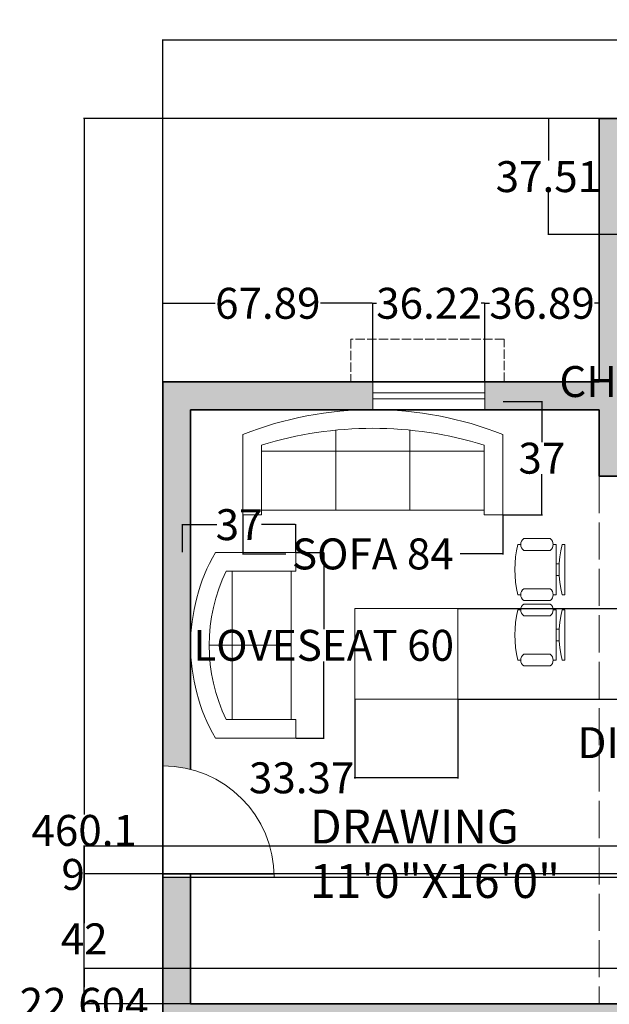
# Model space of a CAD drawing. Units: inches. Extents: x 143 to 746, y -392 to 145.
# Tile 2 of 6: x 143 to 334, y -173 to 145. Entities that reach past the tile are written whole.
import ezdxf

# ---------------------------------------------------------------- set-up
doc = ezdxf.new("R2010")
doc.units = ezdxf.units.IN
doc.header["$MEASUREMENT"] = 0
doc.linetypes.add('ACAD_ISO02W100', pattern=[15, 12, -3])
for name, color, linetype, lineweight in [('A-ANNO-DIMS', 2, 'Continuous', 18), ('A-AREA-IDEN', 7, 'Continuous', 20), ('A-DOOR', 3, 'Continuous', 18), ('A-FURN', 8, 'Continuous', 18), ('A-GLAZ', 4, 'Continuous', 18), ('A-GLAZ-OVHD', 4, 'ACAD_ISO02W100', 13), ('A-WALL', 7, 'Continuous', 35), ('A-WALL-OVHD', 7, 'ACAD_ISO02W100', 18)]:
    doc.layers.add(name, color=color, linetype=linetype, lineweight=lineweight)
doc.layers.add('A-WALL-PATT', color=252, linetype='Continuous', lineweight=13, true_color=0x939598)
doc.styles.get("Standard").update_dxf_attribs({"font": 'arial.ttf'})
doc.dimstyles.get("Standard").update_dxf_attribs({"dimtxt": 10, "dimasz": 0.18, "dimexe": 0.18, "dimexo": 0.0625, "dimgap": 0.09, "dimtad": 0, "dimtih": 1, "dimtoh": 1, "dimdec": 0, "dimzin": 0, "dimdsep": 46, "dimlunit": 3, "dimtxsty": 'Standard', "dimcen": 0.09, "dimadec": 0, "dimazin": 0, "dimtfac": 1, "dimtdec": 0, "dimtofl": 0, "dimtmove": 0, "dimatfit": 3, "dimfxl": 1, "dimtolj": 1, "dimtzin": 0, "dimarcsym": 0})

# ---------------------------------------------------------------- blocks, each defined once
blk = doc.blocks.new('Sofa - Roundback 7 ft.')
for p, q in [((-12.00002, -32.4421), (-12.00003, -6.5971)), ((11.99997, -32.4421), (11.99998, -6.5971)), ((-36.000027, -34), (-36.000027, -11.4696)), ((35.99998, -34), (35.99998, -11.4696)), ((-35.999844, -13.3819), (35.9998, -13.3819)), ((-36.000027, -32.4421), (35.99998, -32.4421))]:
    blk.add_line(p, q)
for points in [[(-36.000027, -34), (-42.000027, -34), (-42.000027, -8)], [(41.99998, -8), (41.99998, -34), (35.99998, -34)]]:
    blk.add_lwpolyline(points)
for centre, radius, start, end in [((0, -114.25), 114.25, 68.43141, 111.5686), ((-0.00001, -127.1968), 121.1968, 72.72033, 107.2797)]:
    blk.add_arc(centre, radius, start, end)
blk = doc.blocks.new('Sofa - Roundback Loveseat 5 ft.')
for p, q in [((0, -32.44198), (0, -5.99998)), ((-24, -33.99998), (-24, -11.46958)), ((24.00004, -33.99998), (24.00004, -11.46958)), ((-23.9998, -13.38178), (23.99986, -13.38178)), ((-24, -32.44198), (24.00004, -32.44198))]:
    blk.add_line(p, q)
for points in [[(-24, -33.99998), (-30, -33.99998), (-30, -7.99998)], [(30.00004, -7.99998), (30.00004, -33.99998), (24.00004, -33.99998)]]:
    blk.add_lwpolyline(points)
for centre, radius, start, end in [((0, -60.24998), 60.24998, 60.13715, 119.8628), ((0, -61.38438), 55.38444, 64.32083, 115.6792)]:
    blk.add_arc(centre, radius, start, end)
blk = doc.blocks.new('Chair - Desk')
for p, q in [((-8.5, 0), (-8.5, -1)), ((-8.5, 0), (8.5, 0)), ((8.5, 0), (8.5, -1)), ((-8.5, -3), (-8.5, -4)), ((-8.5, -3), (8.5, -3)), ((-2, -3), (-2, -1.9355)), ((2, -1.9576), (2, -3)), ((8.5, -3), (8.5, -4)), ((-10.5, -5), (-10.5, -14)), ((-6.5, -14), (-6.5, -5)), ((6.5, -5), (6.5, -14)), ((10.5, -14), (10.5, -5)), ((-8.5, -15), (-8.5, -16)), ((8.5, -15), (8.5, -16))]:
    blk.add_line(p, q)
for centre, radius, start, end in [((0, 34.625), 36.625, 256.5803, 283.4197), ((-8.5, -6.5), 2.5, 36.8699, 143.1301), ((8.5, -6.5), 2.5, 36.8699, 143.1301), ((-8.5, -12.5), 2.5, 216.8699, 323.1301), ((0, 19.625), 36.625, 256.5803, 283.4197), ((8.5, -12.5), 2.5, 216.8699, 323.1301)]:
    blk.add_arc(centre, radius, start, end)
blk = doc.blocks.new('DOOR-SINGLE-36IN')
for p, q in [((36, 36), (0, 36)), ((36, 35), (0, 35))]:
    blk.add_line(p, q)
blk.add_arc((36, 36), 36, 180, 270)
blk = doc.blocks.new('WINDOW-SHADE-49IN')
at = {"ltscale": 0.25}
for p, q in [((49.48, 13.79), (0, 13.79)), ((0, 13.79), (0, 0)), ((49.48, 0), (49.48, 13.79))]:
    blk.add_line(p, q, dxfattribs=at)
blk = doc.blocks.new('*D18')
at = {"layer": 'A-ANNO-DIMS', "color": 0, "lineweight": -2, "transparency": 16777216}
for p, q in [((426.49, 40.22), (410.54, 28.71)), ((428.36, 37.94), (426.53, 40.48)), ((412.12, 26.22), (410.29, 28.75)), ((410.25, 28.5), (410.07, 28.5)), ((410.4, 28.6), (410.25, 28.5))]:
    blk.add_line(p, q, dxfattribs=at)
at = {"layer": 'A-ANNO-DIMS', "color": 0, "transparency": 16777216}
for points in [[(426.47, 40.25), (426.51, 40.2), (426.64, 40.33)], [(410.53, 28.73), (410.56, 28.68), (410.4, 28.6)]]:
    blk.add_solid(points, dxfattribs=at)
at = {"layer": 'Defpoints', "color": 0, "transparency": 16777216}
for p in [(428.4, 37.89), (410.4, 28.6), (412.16, 26.17)]:
    blk.add_point(p, dxfattribs=at)
at = {"layer": 'A-ANNO-DIMS', "color": 0, "transparency": 16777216, "insert": (362.03, 28.5), "char_height": 10, "attachment_point": 5}
blk.add_mtext('\\A1;CHAIR 20 TYP.', dxfattribs=at)
blk = doc.blocks.new('*D28')
at = {"layer": 'A-ANNO-DIMS', "color": 0, "lineweight": -2, "transparency": 16777216}
for p, q in [((215.43, -14.67), (215.43, -27.39)), ((299.43, -14.67), (299.43, -27.39)), ((215.61, -27.21), (229.26, -27.21)), ((299.25, -27.21), (285.59, -27.21))]:
    blk.add_line(p, q, dxfattribs=at)
at = {"layer": 'A-ANNO-DIMS', "color": 0, "transparency": 16777216}
for points in [[(215.61, -27.18), (215.61, -27.24), (215.43, -27.21)], [(299.25, -27.18), (299.25, -27.24), (299.43, -27.21)]]:
    blk.add_solid(points, dxfattribs=at)
at = {"layer": 'Defpoints', "color": 0, "transparency": 16777216}
for p in [(215.43, -14.61), (299.43, -14.61), (299.43, -27.21)]:
    blk.add_point(p, dxfattribs=at)
at = {"layer": 'A-ANNO-DIMS', "color": 0, "transparency": 16777216, "insert": (257.43, -27.21), "char_height": 10, "attachment_point": 5}
blk.add_mtext('\\A1;SOFA 84', dxfattribs=at)
blk = doc.blocks.new('*D29')
at = {"layer": 'A-ANNO-DIMS', "color": 0, "lineweight": -2, "transparency": 16777216}
for p, q in [((299.49, 22.06), (312.21, 22.06)), ((312.03, 21.88), (312.03, 8.92)), ((312.03, -14.43), (312.03, -1.47)), ((299.49, -14.61), (312.21, -14.61))]:
    blk.add_line(p, q, dxfattribs=at)
at = {"layer": 'A-ANNO-DIMS', "color": 0, "transparency": 16777216}
for points in [[(312, 21.88), (312.06, 21.88), (312.03, 22.06)], [(312, -14.43), (312.06, -14.43), (312.03, -14.61)]]:
    blk.add_solid(points, dxfattribs=at)
at = {"layer": 'Defpoints', "color": 0, "transparency": 16777216}
for p in [(299.43, 22.06), (312.03, 22.06), (299.43, -14.61)]:
    blk.add_point(p, dxfattribs=at)
at = {"layer": 'A-ANNO-DIMS', "color": 0, "transparency": 16777216, "insert": (312.03, 3.73), "char_height": 10, "attachment_point": 5}
blk.add_mtext('\\A1;37', dxfattribs=at)
blk = doc.blocks.new('*D30')
at = {"layer": 'A-ANNO-DIMS', "color": 0, "lineweight": -2, "transparency": 16777216}
for p, q in [((232.6, -26.75), (241.72, -26.75)), ((241.54, -26.93), (241.54, -51.48)), ((241.54, -86.57), (241.54, -62.01)), ((232.6, -86.75), (241.72, -86.75))]:
    blk.add_line(p, q, dxfattribs=at)
at = {"layer": 'A-ANNO-DIMS', "color": 0, "transparency": 16777216}
for points in [[(241.51, -26.93), (241.57, -26.93), (241.54, -26.75)], [(241.51, -86.57), (241.57, -86.57), (241.54, -86.75)]]:
    blk.add_solid(points, dxfattribs=at)
at = {"layer": 'Defpoints', "color": 0, "transparency": 16777216}
for p in [(232.54, -26.75), (241.54, -26.75), (232.54, -86.75)]:
    blk.add_point(p, dxfattribs=at)
at = {"layer": 'A-ANNO-DIMS', "color": 0, "transparency": 16777216, "insert": (241.54, -56.75), "char_height": 10, "attachment_point": 5}
blk.add_mtext('\\A1;LOVESEAT 60', dxfattribs=at)
blk = doc.blocks.new('*D31')
at = {"layer": 'A-ANNO-DIMS', "color": 0, "lineweight": -2, "transparency": 16777216}
for p, q in [((195.87, -26.68), (195.87, -17.57)), ((196.05, -17.75), (206.96, -17.75)), ((232.36, -17.75), (221.45, -17.75)), ((232.54, -26.68), (232.54, -17.57))]:
    blk.add_line(p, q, dxfattribs=at)
at = {"layer": 'A-ANNO-DIMS', "color": 0, "transparency": 16777216}
for points in [[(196.05, -17.72), (196.05, -17.78), (195.87, -17.75)], [(232.36, -17.72), (232.36, -17.78), (232.54, -17.75)]]:
    blk.add_solid(points, dxfattribs=at)
at = {"layer": 'Defpoints', "color": 0, "transparency": 16777216}
for p in [(195.87, -17.75), (195.87, -26.75), (232.54, -26.75)]:
    blk.add_point(p, dxfattribs=at)
at = {"layer": 'A-ANNO-DIMS', "color": 0, "transparency": 16777216, "insert": (214.2, -17.75), "char_height": 10, "attachment_point": 5}
blk.add_mtext('\\A1;37', dxfattribs=at)
blk = doc.blocks.new('*D32')
at = {"layer": 'A-ANNO-DIMS', "color": 0, "lineweight": -2, "transparency": 16777216}
for p, q in [((383.18, -42.7), (369.41, -42.7)), ((369.59, -42.88), (369.59, -82.94)), ((369.59, -133.52), (369.59, -93.46)), ((383.18, -133.7), (369.41, -133.7))]:
    blk.add_line(p, q, dxfattribs=at)
at = {"layer": 'A-ANNO-DIMS', "color": 0, "transparency": 16777216}
for points in [[(369.56, -42.88), (369.62, -42.88), (369.59, -42.7)], [(369.56, -133.52), (369.62, -133.52), (369.59, -133.7)]]:
    blk.add_solid(points, dxfattribs=at)
at = {"layer": 'Defpoints', "color": 0, "transparency": 16777216}
for p in [(383.24, -42.7), (369.59, -133.7), (383.24, -133.7)]:
    blk.add_point(p, dxfattribs=at)
at = {"layer": 'A-ANNO-DIMS', "color": 0, "transparency": 16777216, "insert": (369.59, -88.2), "char_height": 10, "attachment_point": 5}
blk.add_mtext('\\A1;DINING SET 91', dxfattribs=at)
blk = doc.blocks.new('*D43')
at = {"layer": 'A-ANNO-DIMS', "color": 0, "lineweight": -2, "transparency": 16777216}
for p, q in [((189.54, 28.45), (189.54, 139.06)), ((189.72, 138.88), (423.22, 138.88)), ((679.36, 138.88), (445.86, 138.88)), ((679.54, 31.45), (679.54, 139.06))]:
    blk.add_line(p, q, dxfattribs=at)
at = {"layer": 'A-ANNO-DIMS', "color": 0, "transparency": 16777216}
for points in [[(189.72, 138.91), (189.72, 138.85), (189.54, 138.88)], [(679.36, 138.91), (679.36, 138.85), (679.54, 138.88)]]:
    blk.add_solid(points, dxfattribs=at)
at = {"layer": 'Defpoints', "color": 0, "transparency": 16777216}
for p in [(679.54, 138.88), (679.54, 31.39), (189.54, 28.39)]:
    blk.add_point(p, dxfattribs=at)
at = {"layer": 'A-ANNO-DIMS', "color": 0, "transparency": 16777216, "insert": (434.54, 138.88), "char_height": 10, "attachment_point": 5}
blk.add_mtext('\\A1;490', dxfattribs=at)
blk = doc.blocks.new('*D44')
at = {"layer": 'A-ANNO-DIMS', "color": 0, "lineweight": -2, "transparency": 16777216}
for p, q in [((189.6, -131.67), (718.91, -131.67)), ((718.73, -131.85), (718.73, -146.94)), ((718.73, -172.43), (718.73, -157.34)), ((198.6, -172.61), (718.91, -172.61))]:
    blk.add_line(p, q, dxfattribs=at)
at = {"layer": 'A-ANNO-DIMS', "color": 0, "transparency": 16777216}
for points in [[(718.7, -131.85), (718.76, -131.85), (718.73, -131.67)], [(718.7, -172.43), (718.76, -172.43), (718.73, -172.61)]]:
    blk.add_solid(points, dxfattribs=at)
at = {"layer": 'Defpoints', "color": 0, "transparency": 16777216}
for p in [(189.54, -131.67), (718.73, -131.67), (198.54, -172.61)]:
    blk.add_point(p, dxfattribs=at)
at = {"layer": 'A-ANNO-DIMS', "color": 0, "transparency": 16777216, "insert": (718.73, -152.14), "char_height": 10, "attachment_point": 5}
blk.add_mtext('\\A1;40.935', dxfattribs=at)
blk = doc.blocks.new('*D45')
at = {"layer": 'A-ANNO-DIMS', "color": 0, "lineweight": -2, "transparency": 16777216}
for p, q in [((330.48, 113.48), (163.96, 113.48)), ((164.14, 113.3), (164.14, -111.37)), ((164.14, -346.43), (164.14, -121.76)), ((189.48, -346.61), (163.96, -346.61))]:
    blk.add_line(p, q, dxfattribs=at)
at = {"layer": 'A-ANNO-DIMS', "color": 0, "transparency": 16777216}
for points in [[(164.11, 113.3), (164.17, 113.3), (164.14, 113.48)], [(164.11, -346.43), (164.17, -346.43), (164.14, -346.61)]]:
    blk.add_solid(points, dxfattribs=at)
at = {"layer": 'Defpoints', "color": 0, "transparency": 16777216}
for p in [(164.14, 113.48), (330.54, 113.48), (189.54, -346.61)]:
    blk.add_point(p, dxfattribs=at)
at = {"layer": 'A-ANNO-DIMS', "color": 0, "transparency": 16777216, "insert": (164.14, -116.56), "char_height": 10, "attachment_point": 5}
blk.add_mtext('\\A1;460.1', dxfattribs=at)
blk = doc.blocks.new('*D46')
at = {"layer": 'A-ANNO-DIMS', "color": 0, "lineweight": -2, "transparency": 16777216}
for p, q in [((189.54, 28.45), (189.54, 53.97)), ((189.72, 53.79), (206.48, 53.79)), ((257.25, 53.79), (240.48, 53.79)), ((257.43, 28.45), (257.43, 53.97))]:
    blk.add_line(p, q, dxfattribs=at)
at = {"layer": 'A-ANNO-DIMS', "color": 0, "transparency": 16777216}
for points in [[(189.72, 53.82), (189.72, 53.76), (189.54, 53.79)], [(257.25, 53.82), (257.25, 53.76), (257.43, 53.79)]]:
    blk.add_solid(points, dxfattribs=at)
at = {"layer": 'Defpoints', "color": 0, "transparency": 16777216}
for p in [(257.43, 53.79), (189.54, 28.39), (257.43, 28.39)]:
    blk.add_point(p, dxfattribs=at)
at = {"layer": 'A-ANNO-DIMS', "color": 0, "transparency": 16777216, "insert": (223.48, 53.79), "char_height": 10, "attachment_point": 5}
blk.add_mtext('\\A1;67.89', dxfattribs=at)
blk = doc.blocks.new('*D47')
at = {"layer": 'A-ANNO-DIMS', "color": 0, "lineweight": -2, "transparency": 16777216}
for p, q in [((257.43, 28.45), (257.43, 53.97)), ((257.61, 53.79), (258.63, 53.79)), ((293.46, 53.79), (292.44, 53.79)), ((293.64, 28.45), (293.64, 53.97))]:
    blk.add_line(p, q, dxfattribs=at)
at = {"layer": 'A-ANNO-DIMS', "color": 0, "transparency": 16777216}
for points in [[(257.61, 53.82), (257.61, 53.76), (257.43, 53.79)], [(293.46, 53.82), (293.46, 53.76), (293.64, 53.79)]]:
    blk.add_solid(points, dxfattribs=at)
at = {"layer": 'Defpoints', "color": 0, "transparency": 16777216}
for p in [(293.64, 53.79), (257.43, 28.39), (293.64, 28.39)]:
    blk.add_point(p, dxfattribs=at)
at = {"layer": 'A-ANNO-DIMS', "color": 0, "transparency": 16777216, "insert": (275.54, 53.79), "char_height": 10, "attachment_point": 5}
blk.add_mtext('\\A1;36.22', dxfattribs=at)
blk = doc.blocks.new('*D48')
at = {"layer": 'A-ANNO-DIMS', "color": 0, "lineweight": -2, "transparency": 16777216}
for p, q in [((293.64, 28.45), (293.64, 53.97)), ((293.82, 53.79), (295.12, 53.79)), ((330.36, 53.79), (329.06, 53.79)), ((330.54, 28.45), (330.54, 53.97))]:
    blk.add_line(p, q, dxfattribs=at)
at = {"layer": 'A-ANNO-DIMS', "color": 0, "transparency": 16777216}
for points in [[(293.82, 53.82), (293.82, 53.76), (293.64, 53.79)], [(330.36, 53.82), (330.36, 53.76), (330.54, 53.79)]]:
    blk.add_solid(points, dxfattribs=at)
at = {"layer": 'Defpoints', "color": 0, "transparency": 16777216}
for p in [(330.54, 53.79), (293.64, 28.39), (330.54, 28.39)]:
    blk.add_point(p, dxfattribs=at)
at = {"layer": 'A-ANNO-DIMS', "color": 0, "transparency": 16777216, "insert": (312.09, 53.79), "char_height": 10, "attachment_point": 5}
blk.add_mtext('\\A1;36.89', dxfattribs=at)
blk = doc.blocks.new('*D50')
at = {"layer": 'A-ANNO-DIMS', "color": 0, "lineweight": -2, "transparency": 16777216}
for p, q in [((339.48, 113.48), (313.96, 113.48)), ((314.14, 113.3), (314.14, 99.92)), ((314.14, 76.15), (314.14, 89.52)), ((339.48, 75.97), (313.96, 75.97))]:
    blk.add_line(p, q, dxfattribs=at)
at = {"layer": 'A-ANNO-DIMS', "color": 0, "transparency": 16777216}
for points in [[(314.11, 113.3), (314.17, 113.3), (314.14, 113.48)], [(314.11, 76.15), (314.17, 76.15), (314.14, 75.97)]]:
    blk.add_solid(points, dxfattribs=at)
at = {"layer": 'Defpoints', "color": 0, "transparency": 16777216}
for p in [(314.14, 113.48), (339.54, 113.48), (339.54, 75.97)]:
    blk.add_point(p, dxfattribs=at)
at = {"layer": 'A-ANNO-DIMS', "color": 0, "transparency": 16777216, "insert": (314.14, 94.72), "char_height": 10, "attachment_point": 5}
blk.add_mtext('\\A1;37.51', dxfattribs=at)
blk = doc.blocks.new('*D67')
at = {"layer": 'A-ANNO-DIMS', "color": 0, "lineweight": -2, "transparency": 16777216}
for p, q in [((528.48, -121.61), (163.96, -121.61)), ((164.14, -121.79), (164.14, -130.43)), ((528.48, -130.61), (163.96, -130.61)), ((164.14, -130.79), (163.96, -130.79)), ((164.14, -130.61), (164.14, -130.79))]:
    blk.add_line(p, q, dxfattribs=at)
at = {"layer": 'A-ANNO-DIMS', "color": 0, "transparency": 16777216}
for points in [[(164.11, -121.79), (164.17, -121.79), (164.14, -121.61)], [(164.11, -130.43), (164.17, -130.43), (164.14, -130.61)]]:
    blk.add_solid(points, dxfattribs=at)
at = {"layer": 'Defpoints', "color": 0, "transparency": 16777216}
for p in [(528.54, -121.61), (164.14, -130.61), (528.54, -130.61)]:
    blk.add_point(p, dxfattribs=at)
at = {"layer": 'A-ANNO-DIMS', "color": 0, "transparency": 16777216, "insert": (160.58, -130.79), "char_height": 10, "attachment_point": 5}
blk.add_mtext('\\A1;9', dxfattribs=at)
blk = doc.blocks.new('*D68')
at = {"layer": 'A-ANNO-DIMS', "color": 0, "lineweight": -2, "transparency": 16777216}
for p, q in [((251.56, -74.23), (251.56, -99.75)), ((284.93, -74.23), (284.93, -99.75)), ((251.56, -99.57), (251.38, -99.57)), ((284.75, -99.57), (251.74, -99.57))]:
    blk.add_line(p, q, dxfattribs=at)
at = {"layer": 'A-ANNO-DIMS', "color": 0, "transparency": 16777216}
for points in [[(251.74, -99.54), (251.74, -99.6), (251.56, -99.57)], [(284.75, -99.54), (284.75, -99.6), (284.93, -99.57)]]:
    blk.add_solid(points, dxfattribs=at)
at = {"layer": 'Defpoints', "color": 0, "transparency": 16777216}
for p in [(251.56, -74.17), (284.93, -74.17), (251.56, -99.57)]:
    blk.add_point(p, dxfattribs=at)
at = {"layer": 'A-ANNO-DIMS', "color": 0, "transparency": 16777216, "insert": (234.42, -99.57), "char_height": 10, "attachment_point": 5}
blk.add_mtext('\\A1;33.37', dxfattribs=at)
blk = doc.blocks.new('*D69')
at = {"layer": 'A-ANNO-DIMS', "color": 0, "lineweight": -2, "transparency": 16777216}
for p, q in [((284.99, -44.86), (718.91, -44.86)), ((718.73, -45.04), (718.73, -54.32)), ((718.73, -73.99), (718.73, -64.72)), ((284.99, -74.17), (718.91, -74.17))]:
    blk.add_line(p, q, dxfattribs=at)
at = {"layer": 'A-ANNO-DIMS', "color": 0, "transparency": 16777216}
for points in [[(718.7, -45.04), (718.76, -45.04), (718.73, -44.86)], [(718.7, -73.99), (718.76, -73.99), (718.73, -74.17)]]:
    blk.add_solid(points, dxfattribs=at)
at = {"layer": 'Defpoints', "color": 0, "transparency": 16777216}
for p in [(284.93, -44.86), (284.93, -74.17), (718.73, -74.17)]:
    blk.add_point(p, dxfattribs=at)
at = {"layer": 'A-ANNO-DIMS', "color": 0, "transparency": 16777216, "insert": (718.73, -59.52), "char_height": 10, "attachment_point": 5}
blk.add_mtext('\\A1;29.31', dxfattribs=at)
blk = doc.blocks.new('*D70')
at = {"layer": 'A-ANNO-DIMS', "color": 0, "lineweight": -2, "transparency": 16777216}
for p, q in [((645.96, -161.14), (163.96, -161.14)), ((164.14, -161.32), (164.14, -167.24)), ((164.14, -183.56), (164.14, -177.64)), ((645.96, -183.74), (163.96, -183.74))]:
    blk.add_line(p, q, dxfattribs=at)
at = {"layer": 'A-ANNO-DIMS', "color": 0, "transparency": 16777216}
for points in [[(164.11, -161.32), (164.17, -161.32), (164.14, -161.14)], [(164.11, -183.56), (164.17, -183.56), (164.14, -183.74)]]:
    blk.add_solid(points, dxfattribs=at)
at = {"layer": 'Defpoints', "color": 0, "transparency": 16777216}
for p in [(646.02, -161.14), (164.14, -183.74), (646.02, -183.74)]:
    blk.add_point(p, dxfattribs=at)
at = {"layer": 'A-ANNO-DIMS', "color": 0, "transparency": 16777216, "insert": (164.14, -172.44), "char_height": 10, "attachment_point": 5}
blk.add_mtext('\\A1;22.604', dxfattribs=at)
blk = doc.blocks.new('*D75')
at = {"layer": 'A-ANNO-DIMS', "color": 0, "lineweight": -2, "transparency": 16777216}
for p, q in [((528.48, -130.61), (163.96, -130.61)), ((164.14, -130.79), (164.14, -146.5)), ((164.14, -172.43), (164.14, -156.72)), ((528.48, -172.61), (163.96, -172.61))]:
    blk.add_line(p, q, dxfattribs=at)
at = {"layer": 'A-ANNO-DIMS', "color": 0, "transparency": 16777216}
for points in [[(164.11, -130.79), (164.17, -130.79), (164.14, -130.61)], [(164.11, -172.43), (164.17, -172.43), (164.14, -172.61)]]:
    blk.add_solid(points, dxfattribs=at)
at = {"layer": 'Defpoints', "color": 0, "transparency": 16777216}
for p in [(164.14, -130.61), (528.54, -130.61), (528.54, -172.61)]:
    blk.add_point(p, dxfattribs=at)
at = {"layer": 'A-ANNO-DIMS', "color": 0, "transparency": 16777216, "insert": (164.14, -151.61), "char_height": 10, "attachment_point": 5}
blk.add_mtext('\\A1;42', dxfattribs=at)

msp = doc.modelspace()

# ---------------------------------------------------------------- hatches: boundary and pattern name
at = {"layer": 'A-WALL-PATT'}
h = msp.add_hatch(color=256, dxfattribs=at)
h.dxf.hatch_style = 1
h.paths.add_polyline_path([(198.538, 19.3924), (257.4275, 19.3924), (257.4275, 28.3924), (189.538, 28.3924), (189.538, -95.6731, -0.06325422), (198.538, -96.8162)])
h.paths.add_polyline_path([(339.538, 66.969), (471.538, 66.969), (472.538, 66.969), (472.538, 31.3924), (472.538, 6.969), (451.2296, 6.969), (451.2296, -2.031), (472.538, -2.031), (472.538, -82.6076), (544.538, -82.6076), (544.538, -38.6894), (535.538, -38.6894), (535.538, -73.6076), (481.538, -73.6076), (481.538, 22.3924), (498.7149, 22.3924), (498.7149, 31.3924), (481.538, 31.3924), (481.538, 66.969), (481.538, 113.4779), (471.538, 113.4779), (471.538, 75.969), (339.538, 75.969), (339.538, 113.4779), (330.538, 113.4779), (330.538, 66.969), (330.538, 28.3924), (293.6446, 28.3924), (293.6446, 19.3924), (330.538, 19.3924), (330.538, 6.969), (330.538, -2.031), (364.5099, -2.031), (364.5099, 6.969), (339.538, 6.969)])
h.paths.add_polyline_path([(570.63, 31.3924), (544.538, 31.3924), (524.7988, 31.3924), (524.7988, 22.3924), (535.538, 22.3924), (535.538, -9.9696, -0.0761882), (544.538, -8.6878), (544.538, 22.3924), (570.63, 22.3924)])
h.paths.add_polyline_path([(679.538, 31.3924), (618.768, 31.3924), (618.768, 22.3924), (670.538, 22.3924), (670.538, -54.5218), (679.538, -54.5218)])
h.paths.add_polyline_path([(679.538, -90.0753), (670.538, -90.0753), (670.538, -121.6076), (537.538, -121.6076), (528.538, -121.6076), (528.538, -130.6076), (537.538, -130.6076), (670.538, -130.6076), (670.538, -150.8923), (679.538, -150.8923)])
h.paths.add_polyline_path([(679.538, -187.0502), (670.538, -187.0502), (670.538, -232.6076), (636.538, -232.6076, -0.07632083), (635.1562, -241.6076), (670.538, -241.6076), (670.538, -256.599), (679.538, -256.599)])
h.paths.add_polyline_path([(606.538, -232.6076), (537.538, -232.6076), (537.538, -241.6076), (597.538, -241.6076), (597.538, -337.6076), (590.545, -337.6076), (590.545, -346.6076), (679.538, -346.6076), (679.538, -316.1251), (670.538, -316.1251), (670.538, -337.6076), (606.538, -337.6076)])
h.paths.add_polyline_path([(537.538, -181.6076), (537.538, -172.6076), (528.538, -172.6076), (528.538, -209.005), (528.538, -269.6672, -0.07632083), (537.538, -271.0491)])
h.paths.add_polyline_path([(566.8252, -337.6076), (537.538, -337.6076), (537.538, -299.6672), (528.538, -299.6672), (528.538, -337.6076), (513.484, -337.6076), (513.484, -346.6076), (566.8252, -346.6076)])
h.paths.add_polyline_path([(477.1278, -337.6076), (408.538, -337.6076), (408.538, -229.6076), (408.538, -181.6076), (493.5793, -181.6076, -0.06316411), (492.538, -172.6076), (399.538, -172.6076), (399.538, -229.6076), (399.538, -337.6076), (388.659, -337.6076), (388.659, -346.6076), (477.1278, -346.6076)])
h.paths.add_polyline_path([(364.4504, -337.6076), (339.538, -337.6076), (339.538, -301.3371), (330.538, -301.3371), (330.538, -337.6076), (307.2736, -337.6076), (307.2736, -346.6076), (364.4504, -346.6076)])
h.paths.add_polyline_path([(339.538, -229.6076), (399.538, -229.6076), (399.538, -220.6076), (369.1898, -220.6076), (330.538, -220.6076), (330.538, -271.2389, -0.07612824), (339.538, -272.6672)])
h.paths.add_polyline_path([(271.3704, -337.6076), (198.538, -337.6076), (198.538, -181.6076), (339.538, -181.6076), (339.538, -172.6076), (198.538, -172.6076), (198.538, -131.6731), (189.538, -131.6731), (189.538, -346.6076), (271.3704, -346.6076)])

# ---------------------------------------------------------------- linework, layer by layer
at = {"layer": 'A-DOOR'}
msp.add_line((189.538, -131.6731), (189.538, -95.6731), dxfattribs=at)
at = {"layer": 'A-FURN'}
msp.add_lwpolyline([(251.5613, -44.8632), (284.9288, -44.8632), (284.9288, -74.1707), (251.5613, -74.1707)], close=True, dxfattribs=at)
at = {"layer": 'A-GLAZ'}
for p, q in [((257.4275, 23.8924), (257.4275, 28.3924)), ((257.4275, 28.3924), (257.4275, 19.3924)), ((293.6446, 19.3924), (293.6446, 28.3924)), ((293.6446, 24.8924), (257.4275, 24.8924)), ((293.6446, 22.8924), (257.4275, 22.8924))]:
    msp.add_line(p, q, dxfattribs=at)
at = {"layer": 'A-WALL'}
for p, q in [((339.538, 113.4779), (330.538, 113.4779)), ((330.538, 113.4779), (330.538, 66.969)), ((330.538, 28.3924), (330.538, 66.969)), ((330.538, 28.3924), (189.538, 28.3924)), ((189.538, 28.3924), (189.538, -346.6076)), ((189.538, 19.3924), (189.538, -172.6076)), ((198.538, 19.3924), (198.538, -96.8162)), ((330.538, 19.3924), (198.538, 19.3924)), ((330.538, -2.031), (330.538, 19.3924)), ((330.538, 6.969), (330.538, 19.3924)), ((472.538, -2.031), (330.538, -2.031)), ((198.538, -130.6731), (198.538, -172.6076)), ((198.538, -172.6076), (339.538, -172.6076))]:
    msp.add_line(p, q, dxfattribs=at)
at = {"layer": 'A-WALL-OVHD'}
msp.add_line((330.538, -2.031), (330.538, -172.6076), dxfattribs=at)

# ---------------------------------------------------------------- block references
at = {"layer": 'A-DOOR', "rotation": 180}
msp.add_blockref('DOOR-SINGLE-36IN', (225.5381, -95.6727), dxfattribs=at)
at = {"layer": 'A-FURN'}
msp.add_blockref('Sofa - Roundback 7 ft.', (257.4275, 19.3924), dxfattribs=at)
at = {"layer": 'A-FURN', "xscale": 0.9538052522890815, "yscale": 0.9538052522890815, "zscale": 0.9538052522890815, "rotation": 270}
for p in [(319.5144, -32.2761), (319.5144, -53.4091)]:
    msp.add_blockref('Chair - Desk', p, dxfattribs=at)
at = {"layer": 'A-FURN', "rotation": 90}
msp.add_blockref('Sofa - Roundback Loveseat 5 ft.', (198.538, -56.7458), dxfattribs=at)
at = {"layer": 'A-GLAZ-OVHD'}
msp.add_blockref('WINDOW-SHADE-49IN', (250.36, 28.392), dxfattribs=at)

# ---------------------------------------------------------------- texts
at = {"layer": 'A-AREA-IDEN'}
for s, height, p in [('DRAWING', 10.95807, (237.077, -120.7916)), ('11\'0"X16\'0"', 10.958074, (237.077, -138.3948))]:
    msp.add_text(s, height=height, dxfattribs=at).set_placement(p)

# ---------------------------------------------------------------- dimensions: what is measured, and where the dimension line sits
at = {"layer": 'A-ANNO-DIMS'}
for base, p1, p2, override, picture, middle in [((679.538, 138.8779), (189.538, 28.3924), (679.538, 31.3924), {"dimdec": 0, "dimlfac": 1, "dimrnd": 0, "dimzin": 0, "dimdsep": 46, "dimlunit": 2}, '*D43', (434.538, 138.8779)), ((257.4275, 53.7924), (189.538, 28.3924), (257.4275, 28.3924), {"dimdec": 2, "dimlfac": 1, "dimrnd": 0, "dimzin": 0, "dimdsep": 46, "dimlunit": 2}, '*D46', (223.4828, 53.7924)), ((293.6446, 53.7924), (257.4275, 28.3924), (293.6446, 28.3924), {"dimdec": 2, "dimlfac": 1, "dimrnd": 0, "dimzin": 0, "dimdsep": 46, "dimlunit": 2}, '*D47', (275.5361, 53.7924))]:
    dim = msp.add_linear_dim(base=base, p1=p1, p2=p2, dimstyle='Standard', override=override, dxfattribs=at)
    dim.commit()
    dim.dimension.update_dxf_attribs({"geometry": picture, "text_midpoint": middle})
for base, p1, p2, angle, override, picture, middle in [((164.138, 113.4779), (189.538, -346.6076), (330.538, 113.4779), 90, {"dimdec": 1, "dimlfac": 1, "dimrnd": 0, "dimzin": 0, "dimdsep": 46, "dimlunit": 2}, '*D45', (164.138, -116.5649)), ((314.138, 113.4779), (339.538, 75.969), (339.538, 113.4779), 90, {"dimdec": 2, "dimlfac": 1, "dimrnd": 0, "dimzin": 0, "dimdsep": 46, "dimlunit": 2}, '*D50', (314.138, 94.7234)), ((330.538, 53.7924), (293.6446, 28.3924), (330.538, 28.3924), 0, {"dimdec": 2, "dimlfac": 1, "dimrnd": 0, "dimzin": 0, "dimdsep": 46, "dimlunit": 2}, '*D48', (312.0913, 53.7924)), ((312.0275, 22.0591), (299.4275, -14.6076), (299.4275, 22.0591), 90, {"dimdec": 0, "dimlfac": 1, "dimrnd": 0, "dimzin": 0, "dimdsep": 46, "dimlunit": 2}, '*D29', (312.0275, 3.7257)), ((195.8714, -17.7457), (232.538, -26.7457), (195.8714, -26.7457), 180, {"dimdec": 0, "dimlfac": 1, "dimrnd": 0, "dimzin": 0, "dimdsep": 46, "dimlunit": 2}, '*D31', (214.2047, -17.7457)), ((718.7255, -74.1707), (284.9288, -44.8632), (284.9288, -74.1707), 90, {"dimdec": 2, "dimlfac": 1, "dimrnd": 0, "dimzin": 0, "dimdsep": 46, "dimlunit": 2}, '*D69', (718.7255, -59.5169)), ((251.5613, -99.5707), (284.9288, -74.1707), (251.5613, -74.1707), 180, {"dimdec": 2, "dimlfac": 1, "dimrnd": 0, "dimzin": 0, "dimdsep": 46, "dimlunit": 2}, '*D68', (234.4223, -99.5707)), ((164.138, -130.6076), (528.538, -121.6076), (528.538, -130.6076), 90, {"dimdec": 0, "dimlfac": 1, "dimrnd": 0, "dimzin": 0, "dimdsep": 46, "dimlunit": 2}, '*D67', (160.5802, -130.7876)), ((164.138, -130.6076), (528.538, -172.6076), (528.538, -130.6076), 90, {"dimdec": 0, "dimlfac": 1, "dimrnd": 0, "dimzin": 0, "dimdsep": 46, "dimlunit": 2}, '*D75', (164.138, -151.6076)), ((718.72548, -131.67308), (198.53803, -172.6076), (189.53803, -131.67308), 90, {"dimdec": 3, "dimlfac": 1, "dimrnd": 0, "dimzin": 0, "dimdsep": 46, "dimlunit": 2}, '*D44', (718.72548, -152.14034)), ((164.138, -183.7414), (646.0181, -161.1374), (646.0181, -183.7414), 90, {"dimdec": 3, "dimlfac": 1, "dimrnd": 0, "dimzin": 0, "dimdsep": 46, "dimlunit": 2}, '*D70', (164.138, -172.4394))]:
    dim = msp.add_linear_dim(base=base, p1=p1, p2=p2, angle=angle, dimstyle='Standard', override=override, dxfattribs=at)
    dim.commit()
    dim.dimension.update_dxf_attribs({"geometry": picture, "text_midpoint": middle})
for base, p1, p2, angle, text, picture, middle in [((410.3987, 28.6033), (428.3961, 37.8939), (412.1576, 26.1675), 215.834351, 'CHAIR <> TYP.', '*D18', (362.0291, 28.4979)), ((241.538, -26.7457), (232.538, -86.7458), (232.538, -26.7457), 90, 'LOVESEAT <>', '*D30', (241.538, -56.7458)), ((369.5922, -133.6958), (383.2422, -42.6958), (383.2422, -133.6958), 270, 'DINING SET <>', '*D32', (369.5922, -88.1958))]:
    dim = msp.add_linear_dim(base=base, p1=p1, p2=p2, angle=angle, text=text, dimstyle='Standard', override={"dimdec": 0, "dimlfac": 1, "dimrnd": 0, "dimzin": 0, "dimdsep": 46, "dimlunit": 2}, dxfattribs=at)
    dim.commit()
    dim.dimension.update_dxf_attribs({"geometry": picture, "text_midpoint": middle})
dim = msp.add_linear_dim(base=(299.4275, -27.2076), p1=(215.4275, -14.6076), p2=(299.4275, -14.6076), text='SOFA <>', dimstyle='Standard', override={"dimdec": 0, "dimlfac": 1, "dimrnd": 0, "dimzin": 0, "dimdsep": 46, "dimlunit": 2}, dxfattribs=at)
dim.commit()
dim.dimension.update_dxf_attribs({"geometry": '*D28', "text_midpoint": (257.4275, -27.2076)})

doc.saveas('drawing.dxf')
